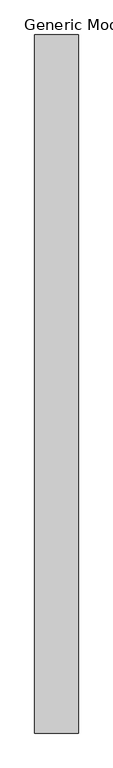
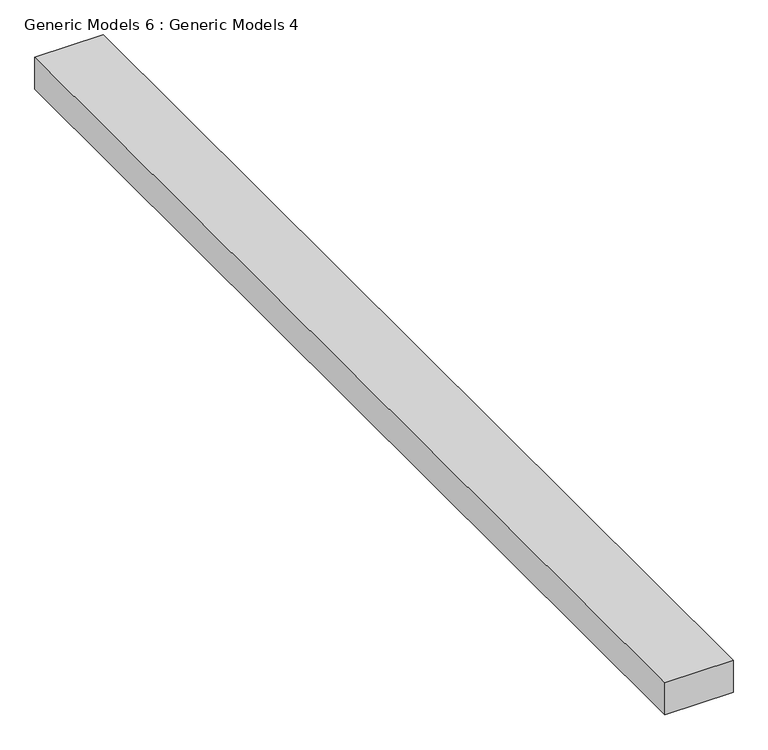
"""IFC4 building model written with IfcOpenShell, lengths in millimetres: proxy geometry, Generic Models 6 : Generic Models 4."""

from ifc_helpers import new_model, si_unit, frame, origin, place, context, project, spatial, polyline, outline, extrude, source, transform, mapped, element, save


def generic_models_6_generic_models_4_f66e2b9f(model_context):
    return source(origin(), model_context, "Body", "SweptSolid", [
        extrude(outline(polyline([(14913.2564936, 13.6653678), (14913.2564936, -12899.9178695), (14106.5361222, -12899.9178695), (14106.5361222, 13.6653678), (14913.2564936, 13.6653678)])), frame((0.0, 0.0, 5892.9645671), z_axis=(0.0, 0.0, 1.0), x_axis=(1.0, 0.0, 0.0)), (0.0, 0.0, 1.0), 398.282593),
    ])


if __name__ == "__main__":
    model = new_model("IFC4")
    model_context = context("Model", 3, world=origin())
    ifc_project = project(units=[si_unit("LENGTHUNIT", "METRE", prefix="MILLI")], contexts=[model_context])
    site = spatial("IfcSite", under=ifc_project)
    building = spatial("IfcBuilding", under=site)
    placement = place(None, origin())
    generic_models_6_generic_models_4_shape = generic_models_6_generic_models_4_f66e2b9f(model_context)
    element("IfcBuildingElementProxy", 1, Name="Generic Models 6 : Generic Models 4", ObjectType="Generic Models 6 : Generic Models 4", at=placement, inside=building, context=model_context, shape_type="MappedRepresentation", body=[
        mapped(generic_models_6_generic_models_4_shape, transform((0.0, 0.0, 0.0), x_axis=(1.0, 0.0, 0.0), y_axis=(0.0, 1.0, 0.0), z_axis=(0.0, 0.0, 1.0))),
    ])
    save(model, "model.ifc")
